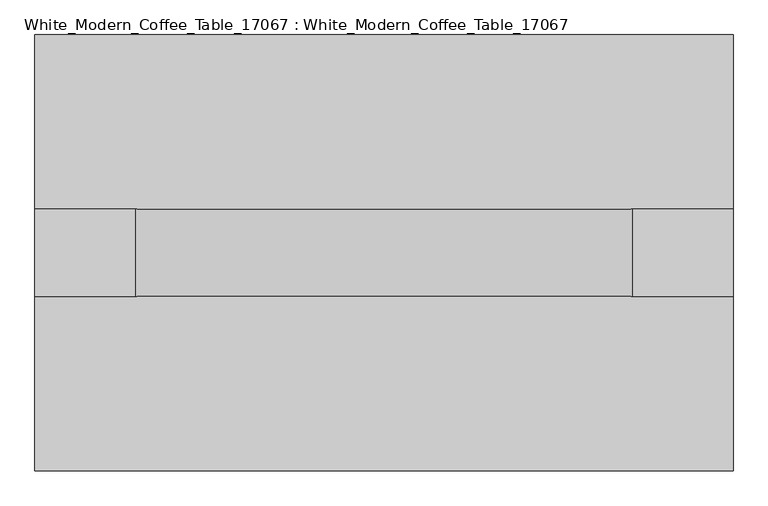
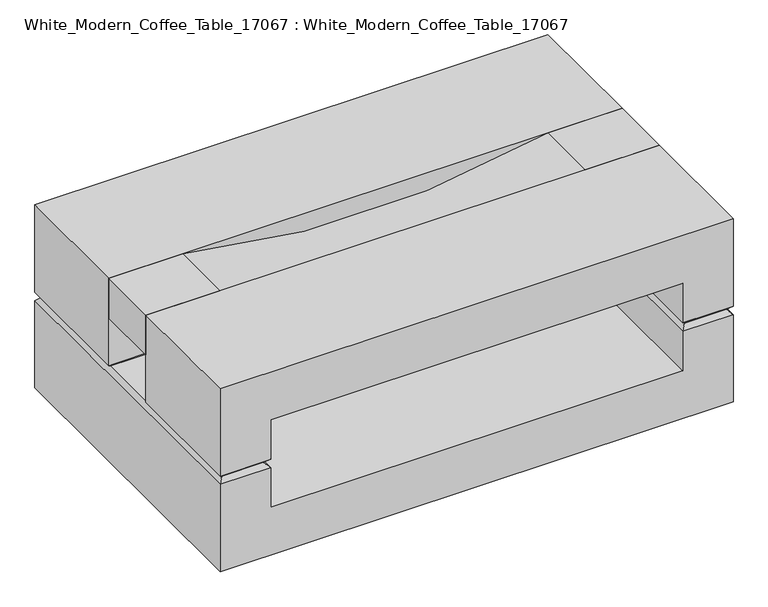
"""IFC4 building model written with IfcOpenShell, lengths in millimetres: furniture geometry, White_Modern_Coffee_Table_17067 : White_Modern_Coffee_Table_17067."""

from ifc_helpers import new_model, si_unit, point, frame, frame_2d, origin, place, context, project, spatial, polyline, circle_curve, trimmed, segment, composite_curve, outline, extrude, faceted_brep, source, transform, mapped, element, save


def white_modern_coffee_table_17067_white_modern_coffee_table_d4aed9ff(model_context):
    return source(origin(), model_context, "Body", "SolidModel", [
        extrude(outline(composite_curve([segment(polyline([(460.0, -434.6), (460.0, -609.6), (360.0, -609.6), (360.0, 609.6), (460.0, 609.6), (460.0, 434.6)]), True, "CONTINUOUS"), segment(trimmed(circle_curve(frame_2d((2323.7716, 0.0)), 1913.7716), [point((460.0, 434.6))], [point((460.0, -434.6))], True, "CARTESIAN"), True, "CONTINUOUS")], self_intersect=False)), frame((0.0, -76.2, 0.0), z_axis=(0.0, 1.0, 0.0), x_axis=(0.0, 0.0, 1.0)), (0.0, 0.0, 1.0), 152.4),
        faceted_brep([(-609.6, -381.0, 0.0), (609.6, -381.0, 0.0), (609.6, -381.0, 219.3933983), (489.6, -381.0, 219.3933983), (489.6, -381.0, 120.0), (-489.6, -381.0, 120.0), (-489.6, -381.0, 219.3933983), (-609.6, -381.0, 219.3933983), (-489.6, 381.0, 120.0), (489.6, 381.0, 120.0), (489.6, 381.0, 219.3933983), (609.6, 381.0, 219.3933983), (609.6, 381.0, 0.0), (-609.6, 381.0, 0.0), (-609.6, 381.0, 219.3933983), (-489.6, 381.0, 219.3933983), (598.9933983, -370.3933983, 230.0), (598.9933983, 370.3933983, 230.0), (500.2066017, 370.3933983, 230.0), (500.2066017, -370.3933983, 230.0), (-500.2066017, -370.3933983, 230.0), (-500.2066017, 370.3933983, 230.0), (-598.9933983, 370.3933983, 230.0), (-598.9933983, -370.3933983, 230.0)], [[[0, 1, 2, 3, 4, 5, 6, 7]], [[8, 9, 10, 11, 12, 13, 14, 15]], [[13, 0, 7, 14]], [[1, 0, 13, 12]], [[1, 12, 11, 2]], [[16, 17, 18, 19]], [[9, 4, 3, 10]], [[5, 4, 9, 8]], [[5, 8, 15, 6]], [[20, 21, 22, 23]], [[14, 7, 23, 22]], [[6, 15, 21, 20]], [[2, 11, 17, 16]], [[10, 3, 19, 18]], [[11, 10, 18, 17]], [[15, 14, 22, 21]], [[3, 2, 16, 19]], [[7, 6, 20, 23]]]),
        faceted_brep([(-489.6, 76.2, 340.0), (489.6, 76.2, 340.0), (489.6, 76.2, 240.6066017), (609.6, 76.2, 240.6066017), (609.6, 76.2, 460.0), (-609.6, 76.2, 460.0), (-609.6, 76.2, 240.6066017), (-489.6, 76.2, 240.6066017), (-609.6, 381.0, 460.0), (609.6, 381.0, 460.0), (609.6, 381.0, 240.6066017), (489.6, 381.0, 240.6066017), (489.6, 381.0, 340.0), (-489.6, 381.0, 340.0), (-489.6, 381.0, 240.6066017), (-609.6, 381.0, 240.6066017), (500.2066017, 370.3933983, 230.0), (598.9933983, 370.3933983, 230.0), (598.9933983, 86.8066017, 230.0), (500.2066017, 86.8066017, 230.0), (-598.9933983, 370.3933983, 230.0), (-500.2066017, 370.3933983, 230.0), (-500.2066017, 86.8066017, 230.0), (-598.9933983, 86.8066017, 230.0)], [[[0, 1, 2, 3, 4, 5, 6, 7]], [[8, 9, 10, 11, 12, 13, 14, 15]], [[5, 8, 15, 6]], [[5, 4, 9, 8]], [[9, 4, 3, 10]], [[16, 17, 18, 19]], [[1, 12, 11, 2]], [[1, 0, 13, 12]], [[13, 0, 7, 14]], [[20, 21, 22, 23]], [[6, 15, 20, 23]], [[14, 7, 22, 21]], [[10, 3, 18, 17]], [[2, 11, 16, 19]], [[11, 10, 17, 16]], [[15, 14, 21, 20]], [[7, 6, 23, 22]], [[3, 2, 19, 18]]]),
        faceted_brep([(-609.6, -76.2, 460.0), (609.6, -76.2, 460.0), (609.6, -76.2, 240.6066017), (489.6, -76.2, 240.6066017), (489.6, -76.2, 340.0), (-489.6, -76.2, 340.0), (-489.6, -76.2, 240.6066017), (-609.6, -76.2, 240.6066017), (-489.6, -381.0, 340.0), (489.6, -381.0, 340.0), (489.6, -381.0, 240.6066017), (609.6, -381.0, 240.6066017), (609.6, -381.0, 460.0), (-609.6, -381.0, 460.0), (-609.6, -381.0, 240.6066017), (-489.6, -381.0, 240.6066017), (598.9933983, -370.3933983, 230.0), (500.2066017, -370.3933983, 230.0), (500.2066017, -86.8066017, 230.0), (598.9933983, -86.8066017, 230.0), (-500.2066017, -370.3933983, 230.0), (-598.9933983, -370.3933983, 230.0), (-598.9933983, -86.8066017, 230.0), (-500.2066017, -86.8066017, 230.0)], [[[0, 1, 2, 3, 4, 5, 6, 7]], [[8, 9, 10, 11, 12, 13, 14, 15]], [[13, 0, 7, 14]], [[1, 0, 13, 12]], [[1, 12, 11, 2]], [[16, 17, 18, 19]], [[9, 4, 3, 10]], [[5, 4, 9, 8]], [[5, 8, 15, 6]], [[20, 21, 22, 23]], [[14, 7, 22, 21]], [[6, 15, 20, 23]], [[2, 11, 16, 19]], [[10, 3, 18, 17]], [[11, 10, 17, 16]], [[15, 14, 21, 20]], [[7, 6, 23, 22]], [[3, 2, 19, 18]]]),
    ])


if __name__ == "__main__":
    model = new_model("IFC4")
    model_context = context("Model", 3, world=origin())
    ifc_project = project(units=[si_unit("LENGTHUNIT", "METRE", prefix="MILLI")], contexts=[model_context])
    site = spatial("IfcSite", under=ifc_project)
    building = spatial("IfcBuilding", under=site)
    placement = place(None, origin())
    white_modern_coffee_table_17067_white_modern_coffee_table_shape = white_modern_coffee_table_17067_white_modern_coffee_table_d4aed9ff(model_context)
    element("IfcFurniture", 1, ObjectType="White_Modern_Coffee_Table_17067 : White_Modern_Coffee_Table_17067", at=placement, inside=building, context=model_context, shape_type="MappedRepresentation", body=[
        mapped(white_modern_coffee_table_17067_white_modern_coffee_table_shape, transform((0.0, 0.0, 0.0), x_axis=(1.0, 0.0, 0.0), y_axis=(0.0, 1.0, 0.0), z_axis=(0.0, 0.0, 1.0))),
    ])
    save(model, "model.ifc")

# Revit data of these elements
# Type "White_Modern_Coffee_Table_17067 : White_Modern_Coffee_Table_17067"
#   White Modern Coffee Table - Wood Width = 0' - 6"
#   White Modern Coffee Table - Width = 2' - 6"
#   White Modern Coffee Table - Length = 4' - 0"
#   White Modern Coffee Table - Wood = White Modern Coffee Table - Wood
#   White Modern Coffee Table - Plastic = White Modern Coffee Table - Plastic
#   Default Elevation = 0
# Element 1 (IfcFurniture, "White_Modern_Coffee_Table_17067 : White_Modern_Coffee_Table_17067")
#   Materials on its faces: "White Modern Coffee Table - Plastic", "White Modern Coffee Table - Wood"
# Materials
#   "White Modern Coffee Table - Wood": class "Generic", colour RGB 120 120 120, transparency 0, Cost = 0
#   "White Modern Coffee Table - Plastic": class "Generic", colour RGB 120 120 120, transparency 0, Cost = 0
